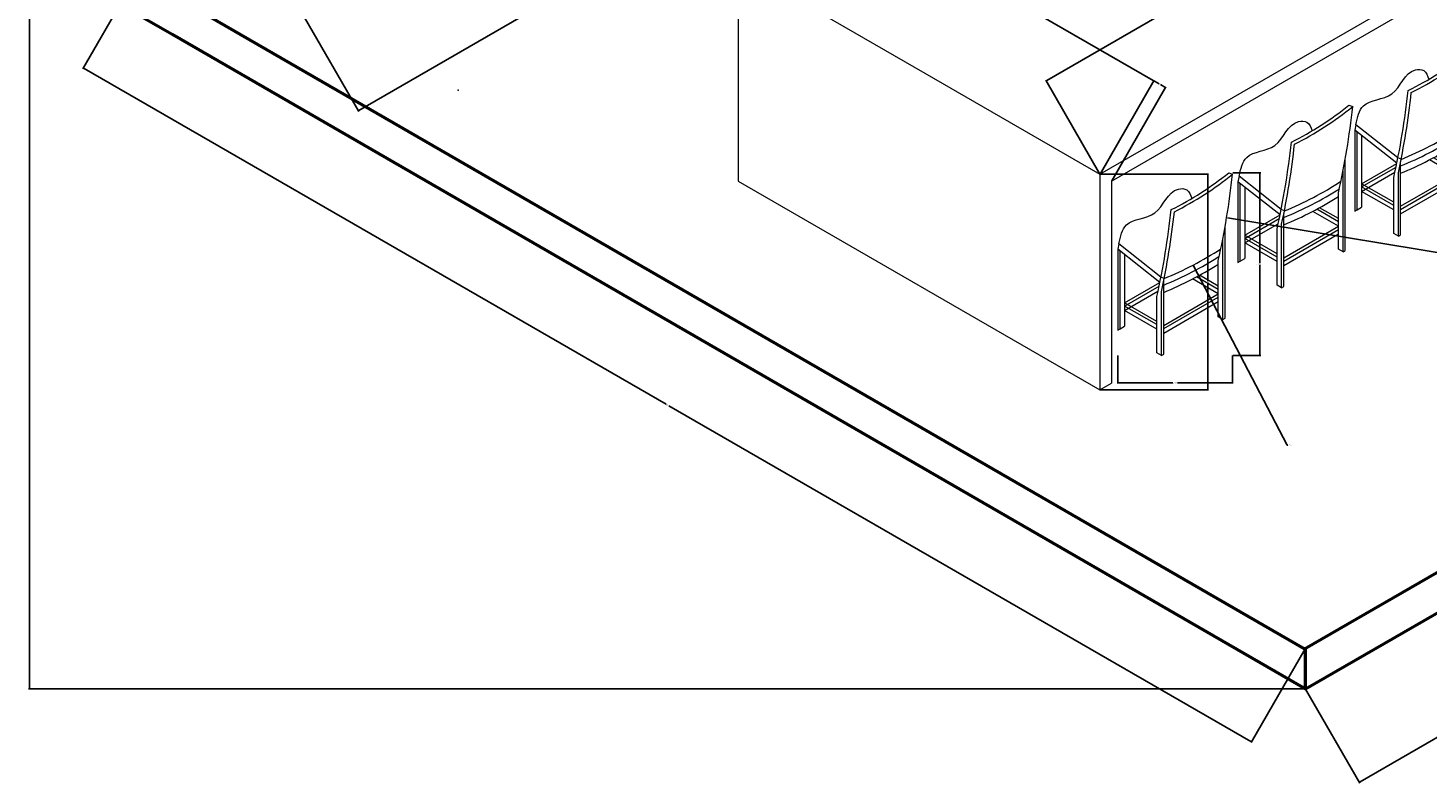
# Model space of a CAD drawing. Units: inches. Extents: x 4150 to 4636, y 2169 to 2592.
# Tile 1 of 8: x 4150 to 4462, y 2169 to 2337. Entities that reach past the tile are written whole.
import ezdxf

# ---------------------------------------------------------------- set-up
doc = ezdxf.new("R2010")
doc.units = ezdxf.units.IN
for name, color, linetype, lineweight in [('A-ANNO-DIMS', 2, 'Continuous', 18), ('A-FURN', 8, 'Continuous', 18), ('A-WALL', 7, 'Continuous', 50)]:
    doc.layers.add(name, color=color, linetype=linetype, lineweight=lineweight)
doc.styles.get("Standard").update_dxf_attribs({"font": 'arial.ttf'})
doc.dimstyles.get("Standard").update_dxf_attribs({"dimtxt": 0.18, "dimasz": 0.18, "dimexe": 0.18, "dimexo": 0.0625, "dimgap": 0.09, "dimtad": 0, "dimtih": 1, "dimtoh": 1, "dimdec": 4, "dimzin": 0, "dimdsep": 46, "dimtxsty": 'Standard', "dimcen": 0.09, "dimadec": 0, "dimazin": 0, "dimtfac": 1, "dimtdec": 4, "dimtofl": 0, "dimtmove": 0, "dimatfit": 3, "dimfxl": 1, "dimtolj": 1, "dimtzin": 0, "dimarcsym": 0})

# ---------------------------------------------------------------- blocks, each defined once
blk = doc.blocks.new('CHAIR')
for p, q in [((4460.61, 2323.17), (4462.07, 2322.64)), ((4459.26, 2268.31), (4459.26, 2302.96)), ((4419.13, 2296.33), (4418.72, 2294.28)), ((4435.02, 2283.82), (4419.13, 2296.33)), ((4458.4, 2267.81), (4458.4, 2298.32)), ((4434.61, 2281.77), (4418.72, 2294.28)), ((4418.72, 2294.28), (4418.72, 2263.74)), ((4419.58, 2264.24), (4419.58, 2293.6)), ((4421.31, 2292.24), (4421.31, 2265.24)), ((4456.67, 2268.81), (4456.67, 2290.03)), ((4421.31, 2274.06), (4434.6, 2281.73)), ((4421.31, 2272.85), (4434.31, 2280.36)), ((4436.24, 2283.27), (4435.02, 2283.82)), ((4436.06, 2254.73), (4436.06, 2282.33)), ((4456.67, 2277.45), (4446.94, 2283.07)), ((4456.67, 2279.13), (4448.46, 2283.88)), ((4456.67, 2280.34), (4449.53, 2284.46)), ((4421.31, 2271.17), (4433.9, 2278.43)), ((4433.46, 2267.05), (4421.31, 2274.06)), ((4433.46, 2255.23), (4433.46, 2276.44)), ((4435.2, 2254.23), (4435.2, 2278.19)), ((4436.06, 2265.55), (4456.67, 2277.45)), ((4436.06, 2264.34), (4456.67, 2276.24)), ((4436.06, 2262.66), (4456.67, 2274.56)), ((4433.46, 2265.84), (4421.31, 2272.85)), ((4433.46, 2264.15), (4421.31, 2271.17)), ((4458.4, 2267.81), (4456.67, 2268.81)), ((4418.72, 2263.74), (4419.58, 2264.24)), ((4419.58, 2264.24), (4421.31, 2265.24)), ((4458.4, 2267.81), (4459.26, 2268.31)), ((4435.2, 2254.23), (4433.46, 2255.23)), ((4435.2, 2254.23), (4436.06, 2254.73))]:
    blk.add_line(p, q)
for centre, radius, start, end in [((4387.22, 2413.69), 116.53, 296.3285, 309.0347), ((4384.96, 2418.26), 122.84, 296.6652, 308.8825), ((4169.51, 2354.34), 294.27, 347.3763, 353.8153), ((4146.35, 2340.95), 294.27, 347.3385, 353.8153), ((4147.53, 2340.19), 294.27, 347.8382, 353.8153), ((4388.03, 2399.21), 127.8, 292.0735, 302.6755), ((4388.03, 2401.62), 127.8, 292.164, 302.9931), ((4387.7, 2396.31), 127.8, 292.2346, 302.6625)]:
    blk.add_arc(centre, radius, start, end)
blk.add_open_spline([(4419.13, 2296.33), (4419.73, 2299.09), (4421.22, 2306.03), (4435.02, 2305.47), (4437.67, 2317.36), (4445.4, 2317.24), (4446.24, 2314.8), (4446.7, 2313.47)], degree=3, knots=[0, 0, 0, 0, 7.695976, 19.302291, 31.993754, 35.157842, 38.967805, 38.967805, 38.967805, 38.967805])
blk = doc.blocks.new('*D16')
at = {"layer": 'A-ANNO-DIMS', "color": 0, "lineweight": -2, "transparency": 16777216}
for p, q in [((4418.24, 2304.64), (4424.45, 2304.64)), ((4424.27, 2304.46), (4424.27, 2284.51)), ((4424.27, 2264.19), (4424.27, 2284.14)), ((4418.24, 2264.01), (4424.45, 2264.01))]:
    blk.add_line(p, q, dxfattribs=at)
at = {"layer": 'A-ANNO-DIMS', "color": 0, "transparency": 16777216}
for points in [[(4424.24, 2304.46), (4424.3, 2304.46), (4424.27, 2304.64)], [(4424.24, 2264.19), (4424.3, 2264.19), (4424.27, 2264.01)]]:
    blk.add_solid(points, dxfattribs=at)
at = {"layer": 'Defpoints', "color": 0, "transparency": 16777216}
for p in [(4418.17, 2304.64), (4424.27, 2304.64), (4418.17, 2264.01)]:
    blk.add_point(p, dxfattribs=at)
at = {"layer": 'A-ANNO-DIMS', "color": 0, "transparency": 16777216, "insert": (4424.27, 2284.33), "char_height": 0.18, "attachment_point": 5}
blk.add_mtext('\\A1;CHAIR 41 TYP.', dxfattribs=at)
blk = doc.blocks.new('*D17')
at = {"layer": 'A-ANNO-DIMS', "color": 0, "lineweight": -2, "transparency": 16777216}
for p, q in [((4392.62, 2263.95), (4392.62, 2257.73)), ((4418.17, 2263.95), (4418.17, 2257.73)), ((4392.8, 2257.91), (4404.87, 2257.91)), ((4417.99, 2257.91), (4405.93, 2257.91))]:
    blk.add_line(p, q, dxfattribs=at)
at = {"layer": 'A-ANNO-DIMS', "color": 0, "transparency": 16777216}
for points in [[(4392.8, 2257.94), (4392.8, 2257.88), (4392.62, 2257.91)], [(4417.99, 2257.94), (4417.99, 2257.88), (4418.17, 2257.91)]]:
    blk.add_solid(points, dxfattribs=at)
at = {"layer": 'Defpoints', "color": 0, "transparency": 16777216}
for p in [(4392.62, 2264.01), (4418.17, 2264.01), (4418.17, 2257.91)]:
    blk.add_point(p, dxfattribs=at)
at = {"layer": 'A-ANNO-DIMS', "color": 0, "transparency": 16777216, "insert": (4405.4, 2257.91), "char_height": 0.18, "attachment_point": 5}
blk.add_mtext('\\A1;26 TYP.', dxfattribs=at)
blk = doc.blocks.new('*D37')
at = {"layer": 'A-ANNO-DIMS', "color": 0, "lineweight": -2, "transparency": 16777216}
for p, q in [((4361.28, 2567.97), (4150.1, 2567.97)), ((4150.28, 2567.79), (4150.28, 2379.06)), ((4150.28, 2189.96), (4150.28, 2378.69)), ((4434.34, 2189.78), (4150.1, 2189.78))]:
    blk.add_line(p, q, dxfattribs=at)
at = {"layer": 'A-ANNO-DIMS', "color": 0, "transparency": 16777216}
for points in [[(4150.25, 2567.79), (4150.31, 2567.79), (4150.28, 2567.97)], [(4150.25, 2189.96), (4150.31, 2189.96), (4150.28, 2189.78)]]:
    blk.add_solid(points, dxfattribs=at)
at = {"layer": 'Defpoints', "color": 0, "transparency": 16777216}
for p in [(4361.34, 2567.97), (4150.28, 2189.78), (4434.4, 2189.78)]:
    blk.add_point(p, dxfattribs=at)
at = {"layer": 'A-ANNO-DIMS', "color": 0, "transparency": 16777216, "insert": (4150.28, 2378.87), "char_height": 0.18, "attachment_point": 5}
blk.add_mtext('\\A1;378.2', dxfattribs=at)
blk = doc.blocks.new('*D38')
at = {"layer": 'A-ANNO-DIMS', "color": 0, "lineweight": -2, "transparency": 16777216}
for p, q in [((4174.25, 2348.68), (4162.2, 2327.79)), ((4162.45, 2327.85), (4292.04, 2253.15)), ((4422.26, 2178.08), (4292.67, 2252.79)), ((4434.37, 2198.73), (4422.33, 2177.84))]:
    blk.add_line(p, q, dxfattribs=at)
at = {"layer": 'A-ANNO-DIMS', "color": 0, "transparency": 16777216}
for points in [[(4162.46, 2327.88), (4162.43, 2327.83), (4162.29, 2327.94)], [(4422.27, 2178.11), (4422.24, 2178.05), (4422.42, 2177.99)]]:
    blk.add_solid(points, dxfattribs=at)
at = {"layer": 'Defpoints', "color": 0, "transparency": 16777216}
for p in [(4174.28, 2348.74), (4162.29, 2327.94), (4434.4, 2198.78)]:
    blk.add_point(p, dxfattribs=at)
at = {"layer": 'A-ANNO-DIMS', "color": 0, "transparency": 16777216, "insert": (4292.35, 2252.97), "char_height": 0.18, "attachment_point": 5}
blk.add_mtext('\\A1;300.25', dxfattribs=at)
blk = doc.blocks.new('*D39')
at = {"layer": 'A-ANNO-DIMS', "color": 0, "lineweight": -2, "transparency": 16777216}
for p, q in [((4608.19, 2290.05), (4620.25, 2269.16)), ((4620, 2269.23), (4533.6, 2219.34)), ((4446.56, 2169.09), (4532.97, 2218.98)), ((4434.43, 2189.73), (4446.49, 2168.84))]:
    blk.add_line(p, q, dxfattribs=at)
at = {"layer": 'A-ANNO-DIMS', "color": 0, "transparency": 16777216}
for points in [[(4619.99, 2269.25), (4620.02, 2269.2), (4620.16, 2269.32)], [(4446.54, 2169.11), (4446.57, 2169.06), (4446.4, 2169)]]:
    blk.add_solid(points, dxfattribs=at)
at = {"layer": 'Defpoints', "color": 0, "transparency": 16777216}
for p in [(4608.16, 2290.1), (4434.4, 2189.78), (4446.4, 2169)]:
    blk.add_point(p, dxfattribs=at)
at = {"layer": 'A-ANNO-DIMS', "color": 0, "transparency": 16777216, "insert": (4533.28, 2219.16), "char_height": 0.18, "attachment_point": 5}
blk.add_mtext('\\A1;200.64', dxfattribs=at)
blk = doc.blocks.new('*D55')
at = {"layer": 'A-ANNO-DIMS', "color": 0, "lineweight": -2, "transparency": 16777216}
for p, q in [((4380.31, 2436.61), (4392.37, 2415.73)), ((4392.12, 2415.79), (4308.21, 2367.35)), ((4223.67, 2318.54), (4307.58, 2366.99)), ((4211.55, 2339.18), (4223.61, 2318.3))]:
    blk.add_line(p, q, dxfattribs=at)
at = {"layer": 'A-ANNO-DIMS', "color": 0, "transparency": 16777216}
for points in [[(4392.11, 2415.82), (4392.14, 2415.77), (4392.28, 2415.88)], [(4223.66, 2318.57), (4223.69, 2318.52), (4223.52, 2318.45)]]:
    blk.add_solid(points, dxfattribs=at)
at = {"layer": 'Defpoints', "color": 0, "transparency": 16777216}
for p in [(4380.28, 2436.67), (4211.52, 2339.24), (4223.52, 2318.45)]:
    blk.add_point(p, dxfattribs=at)
at = {"layer": 'A-ANNO-DIMS', "color": 0, "transparency": 16777216, "insert": (4307.9, 2367.17), "char_height": 0.18, "attachment_point": 5}
blk.add_mtext('\\A1;194.86', dxfattribs=at)
blk = doc.blocks.new('*D66')
at = {"layer": 'A-ANNO-DIMS', "color": 0, "lineweight": -2, "transparency": 16777216}
for p, q in [((4308.14, 2350.86), (4320.2, 2371.75)), ((4320.26, 2371.5), (4360.16, 2348.47)), ((4400.49, 2325.18), (4360.6, 2348.21)), ((4388.68, 2304.36), (4400.74, 2325.25))]:
    blk.add_line(p, q, dxfattribs=at)
at = {"layer": 'A-ANNO-DIMS', "color": 0, "transparency": 16777216}
for points in [[(4320.28, 2371.53), (4320.25, 2371.48), (4320.11, 2371.59)], [(4400.51, 2325.21), (4400.48, 2325.16), (4400.65, 2325.09)]]:
    blk.add_solid(points, dxfattribs=at)
at = {"layer": 'Defpoints', "color": 0, "transparency": 16777216}
for p in [(4308.11, 2350.81), (4400.65, 2325.09), (4388.65, 2304.31)]:
    blk.add_point(p, dxfattribs=at)
at = {"layer": 'A-ANNO-DIMS', "color": 0, "transparency": 16777216, "insert": (4360.38, 2348.34), "char_height": 0.18, "attachment_point": 5}
blk.add_mtext('\\A1;93', dxfattribs=at)
blk = doc.blocks.new('*D67')
at = {"layer": 'A-ANNO-DIMS', "color": 0, "lineweight": -2, "transparency": 16777216}
for p, q in [((4459.63, 2373), (4418.44, 2349.22)), ((4471.75, 2352.36), (4459.7, 2373.25)), ((4376.8, 2325.18), (4418, 2348.96)), ((4388.62, 2304.36), (4376.56, 2325.25))]:
    blk.add_line(p, q, dxfattribs=at)
at = {"layer": 'A-ANNO-DIMS', "color": 0, "transparency": 16777216}
for points in [[(4459.62, 2373.03), (4459.65, 2372.98), (4459.79, 2373.09)], [(4376.79, 2325.21), (4376.82, 2325.16), (4376.65, 2325.09)]]:
    blk.add_solid(points, dxfattribs=at)
at = {"layer": 'Defpoints', "color": 0, "transparency": 16777216}
for p in [(4459.79, 2373.09), (4471.79, 2352.31), (4388.65, 2304.31)]:
    blk.add_point(p, dxfattribs=at)
at = {"layer": 'A-ANNO-DIMS', "color": 0, "transparency": 16777216, "insert": (4418.22, 2349.09), "char_height": 0.18, "attachment_point": 5}
blk.add_mtext('\\A1;96', dxfattribs=at)
blk = doc.blocks.new('*D68')
at = {"layer": 'A-ANNO-DIMS', "color": 0, "lineweight": -2, "transparency": 16777216}
for p, q in [((4388.71, 2304.31), (4412.83, 2304.31)), ((4412.65, 2304.13), (4412.65, 2280.49)), ((4412.65, 2256.49), (4412.65, 2280.12)), ((4388.71, 2256.31), (4412.83, 2256.31))]:
    blk.add_line(p, q, dxfattribs=at)
at = {"layer": 'A-ANNO-DIMS', "color": 0, "transparency": 16777216}
for points in [[(4412.62, 2304.13), (4412.68, 2304.13), (4412.65, 2304.31)], [(4412.62, 2256.49), (4412.68, 2256.49), (4412.65, 2256.31)]]:
    blk.add_solid(points, dxfattribs=at)
at = {"layer": 'Defpoints', "color": 0, "transparency": 16777216}
for p in [(4388.65, 2304.31), (4388.65, 2256.31), (4412.65, 2256.31)]:
    blk.add_point(p, dxfattribs=at)
at = {"layer": 'A-ANNO-DIMS', "color": 0, "transparency": 16777216, "insert": (4412.65, 2280.31), "char_height": 0.18, "attachment_point": 5}
blk.add_mtext('\\A1;48', dxfattribs=at)
blk = doc.blocks.new('*D69')
at = {"layer": 'A-ANNO-DIMS', "color": 0, "lineweight": -2, "transparency": 16777216}
for p, q in [((4388.68, 2304.36), (4400.74, 2325.25)), ((4391.28, 2302.86), (4403.34, 2323.75)), ((4400.8, 2325), (4401.8, 2324.43)), ((4403.09, 2323.68), (4402.1, 2324.26))]:
    blk.add_line(p, q, dxfattribs=at)
at = {"layer": 'A-ANNO-DIMS', "color": 0, "transparency": 16777216}
for points in [[(4400.82, 2325.03), (4400.79, 2324.98), (4400.65, 2325.09)], [(4403.1, 2323.71), (4403.07, 2323.66), (4403.25, 2323.59)]]:
    blk.add_solid(points, dxfattribs=at)
at = {"layer": 'Defpoints', "color": 0, "transparency": 16777216}
for p in [(4403.25, 2323.59), (4388.65, 2304.31), (4391.25, 2302.81)]:
    blk.add_point(p, dxfattribs=at)
at = {"layer": 'A-ANNO-DIMS', "color": 0, "transparency": 16777216, "insert": (4401.95, 2324.34), "char_height": 0.18, "attachment_point": 5}
blk.add_mtext('\\A1;3', dxfattribs=at)
blk = doc.blocks.new('*D75')
at = {"layer": 'A-ANNO-DIMS', "color": 0, "lineweight": -2, "transparency": 16777216}
for p, q in [((4245.64, 2323.02), (4245.82, 2323.02)), ((4245.73, 2322.93), (4245.73, 2323.11)), ((4519.53, 2277.67), (4417.03, 2294.65))]:
    blk.add_line(p, q, dxfattribs=at)
at = {"layer": 'A-ANNO-DIMS', "color": 0, "transparency": 16777216}
blk.add_solid([(4417.03, 2294.68), (4417.02, 2294.62), (4416.85, 2294.68)], dxfattribs=at)
at = {"layer": 'Defpoints', "color": 0, "transparency": 16777216}
for p in [(4245.73, 2323.02), (4416.85, 2294.68)]:
    blk.add_point(p, dxfattribs=at)
at = {"layer": 'A-ANNO-DIMS', "color": 0, "transparency": 16777216, "insert": (4520.08, 2277.67), "char_height": 0.18, "attachment_point": 5}
blk.add_mtext('\\A1;R173.46', dxfattribs=at)
blk = doc.blocks.new('*D76')
at = {"layer": 'A-ANNO-DIMS', "color": 0, "lineweight": -2, "transparency": 16777216}
for p, q in [((4374.44, 2350.89), (4374.62, 2350.89)), ((4374.53, 2350.8), (4374.53, 2350.98)), ((4430.33, 2244.06), (4409.49, 2283.96)), ((4430.51, 2244.06), (4430.33, 2244.06))]:
    blk.add_line(p, q, dxfattribs=at)
at = {"layer": 'A-ANNO-DIMS', "color": 0, "transparency": 16777216}
blk.add_solid([(4409.52, 2283.97), (4409.46, 2283.95), (4409.41, 2284.12)], dxfattribs=at)
at = {"layer": 'Defpoints', "color": 0, "transparency": 16777216}
for p in [(4374.53, 2350.89), (4409.41, 2284.12)]:
    blk.add_point(p, dxfattribs=at)
at = {"layer": 'A-ANNO-DIMS', "color": 0, "transparency": 16777216, "insert": (4430.99, 2244.06), "char_height": 0.18, "attachment_point": 5}
blk.add_mtext('\\A1;R75.33', dxfattribs=at)
blk = doc.blocks.new('*D77')
at = {"layer": 'A-ANNO-DIMS', "color": 0, "lineweight": -2, "transparency": 16777216}
for p, q in [((4425.39, 2387.21), (4425.57, 2387.21)), ((4425.48, 2387.12), (4425.48, 2387.3)), ((4488.19, 2289.8), (4464.77, 2326.18)), ((4488.37, 2289.8), (4488.19, 2289.8))]:
    blk.add_line(p, q, dxfattribs=at)
at = {"layer": 'A-ANNO-DIMS', "color": 0, "transparency": 16777216}
blk.add_solid([(4464.8, 2326.19), (4464.75, 2326.16), (4464.68, 2326.33)], dxfattribs=at)
at = {"layer": 'Defpoints', "color": 0, "transparency": 16777216}
for p in [(4425.48, 2387.21), (4464.68, 2326.33)]:
    blk.add_point(p, dxfattribs=at)
at = {"layer": 'A-ANNO-DIMS', "color": 0, "transparency": 16777216, "insert": (4488.84, 2289.8), "char_height": 0.18, "attachment_point": 5}
blk.add_mtext('\\A1;R72.41', dxfattribs=at)
blk = doc.blocks.new('*D78')
at = {"layer": 'A-ANNO-DIMS', "color": 0, "lineweight": -2, "transparency": 16777216}
for p, q in [((4426.72, 2384.51), (4426.9, 2384.51)), ((4426.81, 2384.42), (4426.81, 2384.6)), ((4486.16, 2292.01), (4464, 2326.55)), ((4486.34, 2292.01), (4486.16, 2292.01))]:
    blk.add_line(p, q, dxfattribs=at)
at = {"layer": 'A-ANNO-DIMS', "color": 0, "transparency": 16777216}
blk.add_solid([(4464.03, 2326.56), (4463.98, 2326.53), (4463.9, 2326.7)], dxfattribs=at)
at = {"layer": 'Defpoints', "color": 0, "transparency": 16777216}
for p in [(4426.81, 2384.51), (4463.9, 2326.7)]:
    blk.add_point(p, dxfattribs=at)
at = {"layer": 'A-ANNO-DIMS', "color": 0, "transparency": 16777216, "insert": (4486.82, 2292.01), "char_height": 0.18, "attachment_point": 5}
blk.add_mtext('\\A1;R68.69', dxfattribs=at)

msp = doc.modelspace()

# ---------------------------------------------------------------- linework, layer by layer
at = {"layer": 'A-FURN'}
for p, q in [((4308.1074, 2350.8064), (4349.6766, 2326.8064)), ((4308.1074, 2350.8064), (4308.1074, 2302.8064)), ((4388.6478, 2304.3064), (4471.7862, 2352.3064)), ((4391.2458, 2302.8064), (4469.1881, 2347.8064)), ((4349.6766, 2326.8064), (4388.6478, 2304.3064)), ((4388.6478, 2304.3064), (4388.6478, 2256.3064)), ((4308.1074, 2302.8064), (4388.6478, 2256.3064)), ((4391.2458, 2302.8064), (4391.2458, 2257.8064)), ((4388.6478, 2256.3064), (4391.2458, 2257.8064))]:
    msp.add_line(p, q, dxfattribs=at)
at = {"layer": 'A-WALL'}
for p, q in [((4174.28, 2348.7364), (4434.204, 2198.6692)), ((4174.28, 2339.9652), (4182.0742, 2335.4652)), ((4182.0742, 2335.4652), (4434.4021, 2189.7836)), ((4434.4021, 2189.7836), (4631.5414, 2303.602)), ((4434.204, 2198.6692), (4600.3645, 2294.602)), ((4434.4021, 2189.7836), (4434.4021, 2198.7836))]:
    msp.add_line(p, q, dxfattribs=at)

# ---------------------------------------------------------------- block references
at = {"layer": 'A-FURN', "xscale": 0.5894434727893052, "yscale": 0.5894434727893052, "zscale": 0.5894434727893052}
for p in [(1840.7944, 961.7822), (1814.7953, 950.3097), (1788.0357, 935.2673)]:
    msp.add_blockref('CHAIR', p, dxfattribs=at)

# ---------------------------------------------------------------- dimensions: what is measured, and where the dimension line sits
at = {"layer": 'A-ANNO-DIMS'}
for base, p1, p2, angle, override, picture, middle in [((4150.28, 2189.7836), (4361.3415, 2567.9652), (4434.4021, 2189.7836), 90, {"dimdec": 1, "dimlfac": 1, "dimrnd": 0, "dimzin": 0, "dimdsep": 46, "dimlunit": 2}, '*D37', (4150.28, 2378.8744)), ((4223.5191, 2318.4518), (4380.2767, 2436.6687), (4211.5191, 2339.2364), 210, {"dimdec": 2, "dimlfac": 1, "dimrnd": 0, "dimzin": 0, "dimdsep": 46, "dimlunit": 2}, '*D55', (4307.8979, 2367.1679)), ((4459.7862, 2373.091), (4388.6478, 2304.3064), (4471.7862, 2352.3064), 30, {"dimdec": 0, "dimlfac": 1, "dimrnd": 0, "dimzin": 0, "dimdsep": 46, "dimlunit": 2}, '*D67', (4418.217, 2349.091)), ((4400.6478, 2325.091), (4308.1074, 2350.8064), (4388.6478, 2304.3064), 330, {"dimdec": 0, "dimlfac": 1, "dimrnd": 0, "dimzin": 0, "dimdsep": 46, "dimlunit": 2}, '*D66', (4360.3776, 2348.341)), ((4162.2937, 2327.9439), (4434.4021, 2198.7836), (4174.28, 2348.7364), 150.037803, {"dimdec": 2, "dimlfac": 1, "dimrnd": 0, "dimzin": 0, "dimdsep": 46, "dimlunit": 2}, '*D38', (4292.3547, 2252.9675)), ((4403.2458, 2323.591), (4388.6478, 2304.3064), (4391.2458, 2302.8064), 330, {"dimdec": 0, "dimlfac": 1, "dimrnd": 0, "dimzin": 0, "dimdsep": 46, "dimlunit": 2}, '*D69', (4401.9468, 2324.341)), ((4412.6478, 2256.3064), (4388.6478, 2304.3064), (4388.6478, 2256.3064), 270, {"dimdec": 0, "dimlfac": 1, "dimrnd": 0, "dimzin": 0, "dimdsep": 46, "dimlunit": 2}, '*D68', (4412.6478, 2280.3064)), ((4446.4021, 2168.999), (4608.1587, 2290.102), (4434.4021, 2189.7836), 210, {"dimdec": 2, "dimlfac": 1, "dimrnd": 0, "dimzin": 0, "dimdsep": 46, "dimlunit": 2}, '*D39', (4533.2804, 2219.1582))]:
    dim = msp.add_linear_dim(base=base, p1=p1, p2=p2, angle=angle, dimstyle='Standard', override=override, dxfattribs=at)
    dim.commit()
    dim.dimension.update_dxf_attribs({"geometry": picture, "text_midpoint": middle})
for center, mpoint, picture, middle in [((4425.4794, 2387.2104), (4464.6759, 2326.3282), '*D77', (4488.8362, 2289.7989)), ((4426.8142, 2384.5135), (4463.904, 2326.699), '*D78', (4486.8179, 2292.0103)), ((4374.5318, 2350.8893), (4409.4062, 2284.1195), '*D76', (4430.9907, 2244.0577)), ((4245.7269, 2323.0174), (4416.8518, 2294.675), '*D75', (4519.5268, 2277.6696))]:
    dim = msp.add_radius_dim(center=center, mpoint=mpoint, dimstyle='Standard', override={"dimdec": 2, "dimlfac": 1, "dimrnd": 0, "dimzin": 0, "dimdsep": 46, "dimlunit": 2}, dxfattribs=at)
    dim.commit()
    dim.dimension.update_dxf_attribs({"geometry": picture, "text_midpoint": middle, "dimtype": 164})
dim = msp.add_linear_dim(base=(4424.2687, 2304.6436), p1=(4418.1735, 2264.0091), p2=(4418.1735, 2304.6436), angle=90, text='CHAIR <> TYP.', dimstyle='Standard', override={"dimdec": 0, "dimlfac": 1, "dimrnd": 0, "dimzin": 0, "dimdsep": 46, "dimlunit": 2}, dxfattribs=at)
dim.commit()
dim.dimension.update_dxf_attribs({"geometry": '*D16', "text_midpoint": (4424.2687, 2284.3263)})
dim = msp.add_linear_dim(base=(4418.1735, 2257.9139), p1=(4392.6194, 2264.0091), p2=(4418.1735, 2264.0091), text='<> TYP.', dimstyle='Standard', override={"dimdec": 0, "dimlfac": 1, "dimrnd": 0, "dimzin": 0, "dimdsep": 46, "dimlunit": 2}, dxfattribs=at)
dim.commit()
dim.dimension.update_dxf_attribs({"geometry": '*D17', "text_midpoint": (4405.3964, 2257.9139)})

doc.saveas('drawing.dxf')
